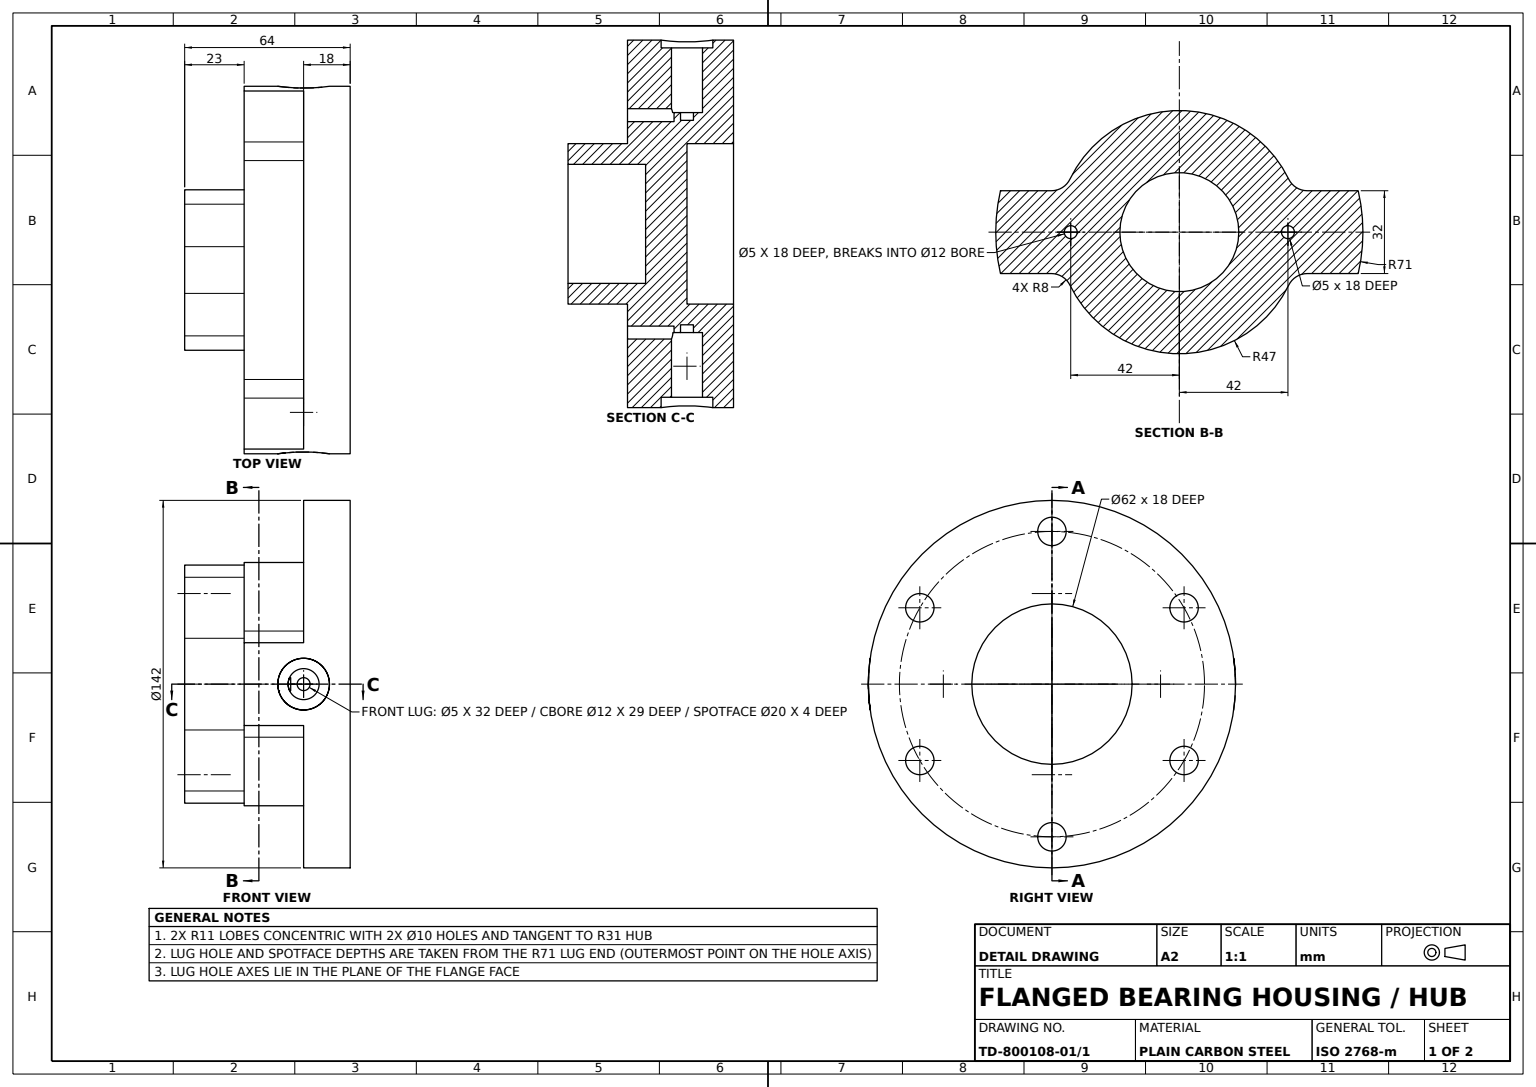
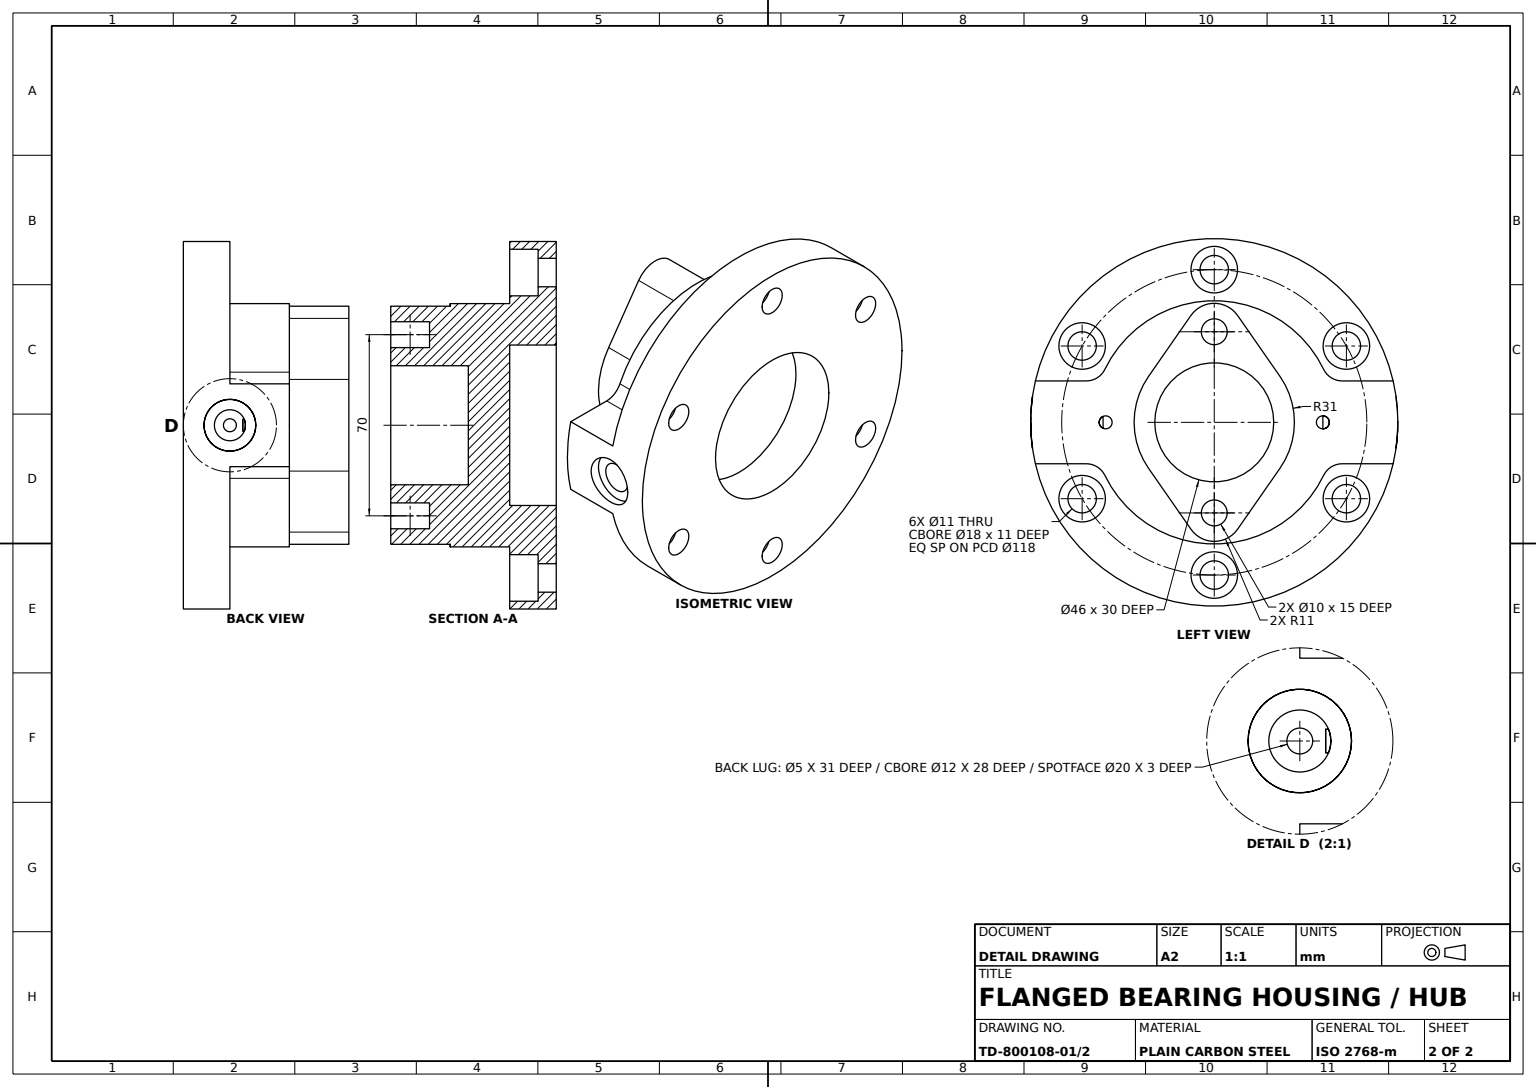
SolidWorks part; units mm, degrees
material "Plain Carbon Steel"
ref_plane "Front Plane" through (0, 0, 0) normal (0, 0, 1) x (1, 0, 0)
ref_plane "Top Plane" through (0, 0, 0) normal (0, 1, 0) x (1, 0, 0)
ref_plane "Right Plane" through (0, 0, 0) normal (1, 0, 0) x (0, 0, -1)
sketch "Flange Sketch" plane through (0, 0, 0) normal (0, 0, 1) x (1, 0, 0)
  circle A0 centre (0, 0) radius 71
  dimension "D1" = 142
extrude "Flange Ø142" add sketch "Flange Sketch" along normal blind 18
sketch "Body Boss Sketch" plane through (0, 0, 18) normal (0, 0, 1) x (1, 0, 0)
  line L1 (-69.1737, 16) -> (-49.4874, 16)
  line L3 (69.1737, -16) -> (49.4874, -16)
  line L6 (49.4874, 16) -> (69.1737, 16)
  line L7 (-49.4874, -16) -> (-69.1737, -16)
  arc A0 (-42.2892, -20.5091) -> (42.2892, -20.5091) centre (0, 0) ccw
  arc A3 (-69.1737, 16) -> (-69.1737, -16) centre (0, 0) ccw
  arc A4 (42.2892, 20.5091) -> (-42.2892, 20.5091) centre (0, 0) ccw
  arc A5 (-42.2892, -20.5091) -> (-49.4874, -16) centre (-49.4874, -24) ccw
  arc A6 (49.4874, -16) -> (42.2892, -20.5091) centre (49.4874, -24) ccw
  arc A7 (49.4874, 16) -> (42.2892, 20.5091) centre (49.4874, 24) cw
  arc A8 (-42.2892, 20.5091) -> (-49.4874, 16) centre (-49.4874, 24) cw
  arc A9 (69.1737, -16) -> (69.1737, 16) centre (0, 0) ccw
  point P19 (44.1928, 16)
  dimension "D1" = 47
  dimension "D3" = 26.8845
  dimension "D4" = 4.5091
  dimension "D2" = 8
  dimension "D5" = 4.5091
extrude "Body Boss With Lugs" add sketch "Body Boss Sketch" along normal blind 23
sketch "Flange Counterbore Sketch" plane through (0, 0, 18) normal (0, 0, 1) x (1, 0, 0)
  line L0 (0, 0) -> (0, 59)
  circle A0 centre (0, 59) radius 9
  circle A1 centre (51.0955, 29.5) radius 9
  circle A2 centre (51.0955, -29.5) radius 9
  circle A3 centre (0, -59) radius 9
  circle A4 centre (-51.0955, -29.5) radius 9
  circle A5 centre (-51.0955, 29.5) radius 9
  dimension "D1" = 59
  dimension "D2" = 18
  dimension "D4" = 29.5
  dimension "D5" = 59
  dimension "D3" = 6
extrude "Flange Counterbores 6x" cut sketch "Flange Counterbore Sketch" against normal blind 11
sketch "Flange Hole Sketch" plane through (0, 0, 18) normal (0, 0, 1) x (1, 0, 0)
  circle A0 centre (0, 59) radius 5.5
  circle A1 centre (51.0955, 29.5) radius 5.5
  circle A2 centre (51.0955, -29.5) radius 5.5
  circle A3 centre (0, -59) radius 5.5
  circle A4 centre (-51.0955, -29.5) radius 5.5
  circle A5 centre (-51.0955, 29.5) radius 5.5
  dimension "D1" = 11
  dimension "D3" = 29.5
  dimension "D4" = 51.0955
  dimension "D2" = 6
extrude "Flange Holes 6xØ11" cut sketch "Flange Hole Sketch" against normal blind 20
sketch "Top Boss Sketch" plane through (0, 0, 41) normal (0, 0, 1) x (1, 0, 0)
  line L0 (0, 0) -> (0, 35)
  line L1 (0, 0) -> (0, -35)
  line L2 (9.0272, -41.2857) -> (25.4402, -17.7143)
  line L3 (-9.0272, -41.2857) -> (-25.4402, -17.7143)
  line L4 (-9.0272, 41.2857) -> (-25.4402, 17.7143)
  line L5 (9.0272, 41.2857) -> (25.4402, 17.7143)
  arc A0 (25.4402, -17.7143) -> (25.4402, 17.7143) centre (0, 0) ccw
  arc A1 (9.0272, 41.2857) -> (-9.0272, 41.2857) centre (0, 35) ccw
  arc A2 (-9.0272, -41.2857) -> (9.0272, -41.2857) centre (0, -35) ccw
  arc A3 (-25.4402, 17.7143) -> (-25.4402, -17.7143) centre (0, 0) ccw
  dimension "D1" = 62
  dimension "D4" = 11
  dimension "D5" = 11
  dimension "D2" = 35
  dimension "D3" = 35
extrude "Top Boss" add sketch "Top Boss Sketch" along normal blind 23
sketch "Bore Sketch" plane through (0, 0, 64) normal (0, 0, 1) x (1, 0, 0)
  circle A0 centre (0, 0) radius 23
  dimension "D1" = 46
extrude "Bore Ø46" cut sketch "Bore Sketch" against normal blind 30
sketch "Top Boss Hole Sketch" plane through (0, 0, 64) normal (0, 0, 1) x (1, 0, 0)
  line L0 (0, 0) -> (0, 35)
  line L1 (0, 0) -> (0, -35)
  circle A0 centre (0, 35) radius 5
  circle A1 centre (0, -35) radius 5
  dimension "D3" = 10
  dimension "D4" = 10
  dimension "D1" = 35
  dimension "D2" = 35
extrude "Top Boss Holes" cut sketch "Top Boss Hole Sketch" against normal blind 15
sketch "Through Bore Sketch" plane through (0, 0, 0) normal (0, 0, -1) x (-1, 0, 0)
  circle A0 centre (0, 0) radius 31
  dimension "D1" = 62
extrude "Through Bore Ø62" cut sketch "Through Bore Sketch" against normal blind 18
sketch "Body Boss Hole Sketch" plane through (0, 0, 41) normal (0, 0, 1) x (1, 0, 0)
  line L0 (0, 0) -> (-42, 0)
  line L1 (0, 0) -> (42, 0)
  circle A0 centre (-42, 0) radius 2.5
  circle A1 centre (42, 0) radius 2.5
  dimension "D3" = 5
  dimension "D4" = 5
  dimension "D1" = 42
  dimension "D2" = 42
extrude "Body Boss Holes" cut sketch "Body Boss Hole Sketch" against normal blind 18
ref_plane "Lug Plane A" through (72, 0, 0) normal (1, 0, 0) x (0, 0, -1)
sketch "Lug A Spot Face Sketch" plane through (72, 0, 0) normal (1, 0, 0) x (0, 0, -1)
  line L0 (-18, 16) -> (-18, -16)
  circle A0 centre (-18, 0) radius 10
  dimension "D1" = 20
extrude "Lug A Spot Face" cut sketch "Lug A Spot Face Sketch" against normal blind 4 contours L0 A0 | L0 A0
sketch "Lug A Hole Ø12 Sketch" plane through (68, 0, 0) normal (1, 0, 0) x (0, 0, -1)
  circle A0 centre (-18, 0) radius 6
  dimension "D1" = 12
extrude "Lug A Hole Ø12" cut sketch "Lug A Hole Ø12 Sketch" against normal blind 25
sketch "Lug A Hole Ø5 Sketch" plane through (43, 0, 0) normal (1, 0, 0) x (0, 0, -1)
  circle A0 centre (-18, 0) radius 2.5
  dimension "D1" = 5
extrude "Lug A Hole Ø5" cut sketch "Lug A Hole Ø5 Sketch" against normal blind 3
ref_plane "Plane2" through (-72, 0, 0) normal (1, 0, 0) x (0, 0, -1)
ref_plane "Plane3" through (-71, 0, 0) normal (1, 0, 0) x (0, 0, -1)
ref_plane "Lug Plane B" through (-71, 0, 0) normal (1, 0, 0) x (0, 0, -1)
sketch "Lug B Spot Face Sketch" plane through (-71, 0, 0) normal (1, 0, 0) x (0, 0, -1)
  circle A0 centre (-18, 0) radius 10
  dimension "D1" = 20
  dimension "D2" = 18
extrude "Lug B Spot Face" cut sketch "Lug B Spot Face Sketch" along normal blind 4
sketch "Lug B Hole Ø12 Sketch" plane through (-67, 0, 0) normal (-1, 0, 0) x (0, 0, 1)
  circle A0 centre (18, 0) radius 6
  dimension "D1" = 12
extrude "Lug B Hole Ø12" cut sketch "Lug B Hole Ø12 Sketch" against normal blind 25
sketch "Lug B Hole Ø5 Sketch" plane through (-42, 0, 0) normal (-1, 0, 0) x (0, 0, 1)
  circle A0 centre (18, 0) radius 2.5
  dimension "D1" = 5
extrude "Lug B Hole Ø5" cut sketch "Lug B Hole Ø5 Sketch" against normal blind 3
